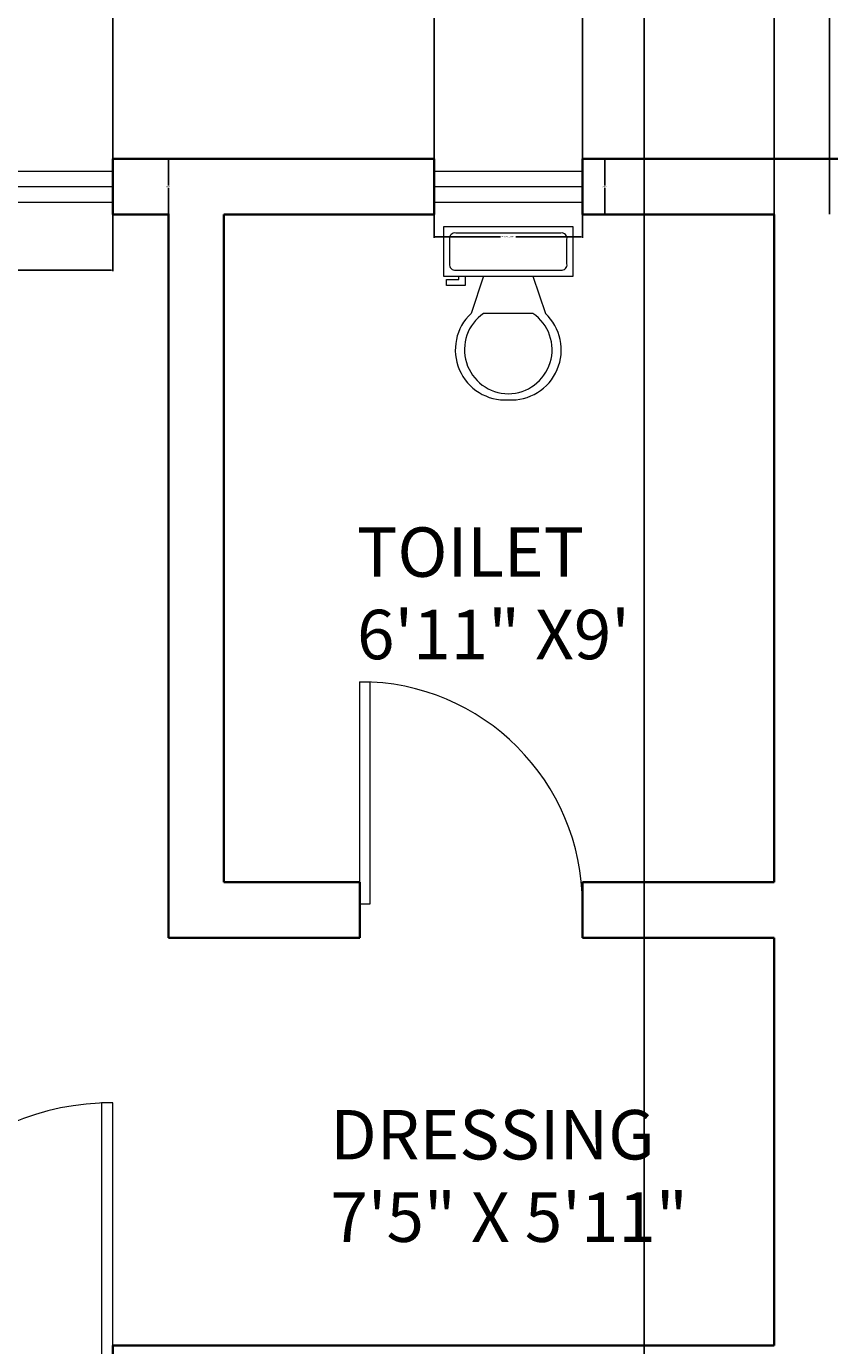
# Model space of a CAD drawing. Units: inches. Extents: x -4843 to -3402, y -164 to 3629.
# Tile 17 of 22: x -4433 to -4303, y 828 to 1042. Entities that reach past the tile are written whole.
import ezdxf

# ---------------------------------------------------------------- set-up
doc = ezdxf.new("R2010")
doc.units = ezdxf.units.IN
for name, color, linetype, lineweight in [('A-ANNO-DIMS', 2, 'Continuous', 18), ('A-AREA-IDEN', 2, 'Continuous', 18), ('doors', 2, 'Continuous', 18), ('toilets', 5, 'Continuous', 18), ('walls', 7, 'Continuous', 35), ('windows', 1, 'Continuous', 18)]:
    doc.layers.add(name, color=color, linetype=linetype, lineweight=lineweight)
doc.styles.get("Standard").update_dxf_attribs({"font": 'arial.ttf'})
doc.dimstyles.get("Standard").update_dxf_attribs({"dimtxt": 0.18, "dimasz": 0.18, "dimexe": 0.18, "dimexo": 0.0625, "dimgap": 0.09, "dimtad": 0, "dimtih": 1, "dimtoh": 1, "dimdec": 4, "dimzin": 0, "dimdsep": 46, "dimtxsty": 'Standard', "dimcen": 0.09, "dimadec": 0, "dimazin": 0, "dimtfac": 1, "dimtdec": 4, "dimtofl": 0, "dimtmove": 0, "dimatfit": 3, "dimfxl": 1, "dimtolj": 1, "dimtzin": 0, "dimarcsym": 0})

# ---------------------------------------------------------------- blocks, each defined once
blk = doc.blocks.new('window')
at = {"layer": 'windows'}
for p, q in [((0, 7), (60, 7)), ((0, 4.5), (60, 4.5)), ((0, 2), (60, 2))]:
    blk.add_line(p, q, dxfattribs=at)
for points in [[(0, 9), (0, 0)], [(60, 0), (60, 9)]]:
    blk.add_lwpolyline(points, dxfattribs=at)
blk = doc.blocks.new('window 2')
at = {"layer": 'windows'}
for p, q in [((0, 8.18), (24, 8.18)), ((0, 5.68), (24, 5.68)), ((0, 3.18), (24, 3.18))]:
    blk.add_line(p, q, dxfattribs=at)
for points in [[(0, 10.18), (0, 1.18)], [(24, 1.18), (24, 10.18)]]:
    blk.add_lwpolyline(points, dxfattribs=at)
blk = doc.blocks.new('*U8')
for p, q in [((0, 0), (0, -6)), ((-40, 0), (-40, -6))]:
    blk.add_line(p, q)
blk.add_lwpolyline([(0, 0), (0, 40), (-1.75, 40), (-1.75, 0)], close=True)
blk.add_arc((0, 0), 40, 90, 180)
blk = doc.blocks.new('*U7')
for p, q in [((0, 0), (0, -6)), ((40, 0), (40, -6))]:
    blk.add_line(p, q)
blk.add_lwpolyline([(0, 0), (0, 40), (1.75, 40), (1.75, 0)], close=True)
blk.add_arc((0, 0), 40, 0, 90)
blk = doc.blocks.new('*U31')
for p, q in [((241.3, -152.4), (241.3, -50.8)), ((-254, -215.9), (-203.2, -215.9)), ((-254, -241.3), (-254, -215.9)), ((-203.2, -215.9), (-203.2, -203.2)), ((-177.8, -203.2), (-177.8, -241.3)), ((-101.6, -203.2), (-152.4, -355.6)), ((101.6, -203.2), (152.4, -355.6)), ((-177.8, -241.3), (-254, -241.3)), ((101.6, -355.6), (-101.6, -355.6))]:
    blk.add_line(p, q)
blk.add_lwpolyline([(266.7, -203.2), (266.7, 0), (-266.7, 0), (-266.7, -203.2)], close=True)
for points in [[(-241.3, -50.8), (-241.3, -152.4)], [(215.9, -25.4), (-215.9, -25.4)], [(-215.9, -177.8), (215.9, -177.8)]]:
    blk.add_lwpolyline(points)
for centre, radius, start, end in [((-219.075, -47.625), 22.45064, 81.8699, 188.1301), ((219.075, -47.625), 22.45064, 351.8699, 98.1301), ((-219.075, -155.575), 22.45064, 171.869898, 278.1301), ((219.075, -155.575), 22.45064, 261.8699, 8.1301), ((-12.12088, -505.93752), 205.61935, 133.01722, 273.38), ((0.94996, -504.77674), 181.02486, 124.50543, 269.7), ((-0.94742, -504.77674), 181.02486, 270.3, 55.4946), ((12.12342, -505.93752), 205.61935, 266.62, 46.9828)]:
    blk.add_arc(centre, radius, start, end)
blk = doc.blocks.new('*D36')
at = {"layer": 'A-ANNO-DIMS', "color": 0, "lineweight": -2, "transparency": 16777216}
for p, q in [((-4478.78, 1011.29), (-4478.78, 1002.17)), ((-4418.78, 1011.29), (-4418.78, 1002.17)), ((-4478.6, 1002.35), (-4450.02, 1002.35)), ((-4418.96, 1002.35), (-4447.55, 1002.35))]:
    blk.add_line(p, q, dxfattribs=at)
at = {"layer": 'A-ANNO-DIMS', "color": 0, "transparency": 16777216}
for points in [[(-4478.6, 1002.38), (-4478.6, 1002.32), (-4478.78, 1002.35)], [(-4418.96, 1002.38), (-4418.96, 1002.32), (-4418.78, 1002.35)]]:
    blk.add_solid(points, dxfattribs=at)
at = {"layer": 'Defpoints', "color": 0, "transparency": 16777216}
for p in [(-4478.78, 1011.35), (-4418.78, 1011.35), (-4418.78, 1002.35)]:
    blk.add_point(p, dxfattribs=at)
at = {"layer": 'A-ANNO-DIMS', "color": 0, "transparency": 16777216, "insert": (-4448.78, 1002.35), "char_height": 0.18, "attachment_point": 5}
blk.add_mtext('\\A1;WINDOW A 60 TYP.', dxfattribs=at)
blk = doc.blocks.new('*D37')
at = {"layer": 'A-ANNO-DIMS', "color": 0, "lineweight": -2, "transparency": 16777216}
for p, q in [((-4418.72, 1020.35), (-4409.6, 1020.35)), ((-4409.78, 1020.17), (-4409.78, 1016.04)), ((-4409.78, 1011.53), (-4409.78, 1015.67)), ((-4418.72, 1011.35), (-4409.6, 1011.35))]:
    blk.add_line(p, q, dxfattribs=at)
at = {"layer": 'A-ANNO-DIMS', "color": 0, "transparency": 16777216}
for points in [[(-4409.81, 1020.17), (-4409.75, 1020.17), (-4409.78, 1020.35)], [(-4409.81, 1011.53), (-4409.75, 1011.53), (-4409.78, 1011.35)]]:
    blk.add_solid(points, dxfattribs=at)
at = {"layer": 'Defpoints', "color": 0, "transparency": 16777216}
for p in [(-4418.78, 1020.35), (-4409.78, 1020.35), (-4418.78, 1011.35)]:
    blk.add_point(p, dxfattribs=at)
at = {"layer": 'A-ANNO-DIMS', "color": 0, "transparency": 16777216, "insert": (-4409.78, 1015.85), "char_height": 0.18, "attachment_point": 5}
blk.add_mtext('\\A1;9 TYP.', dxfattribs=at)
blk = doc.blocks.new('*D40')
at = {"layer": 'A-ANNO-DIMS', "color": 0, "lineweight": -2, "transparency": 16777216}
for p, q in [((-4366.78, 1011.29), (-4366.78, 1007.57)), ((-4342.78, 1011.29), (-4342.78, 1007.57)), ((-4366.6, 1007.75), (-4356.03, 1007.75)), ((-4342.96, 1007.75), (-4353.54, 1007.75))]:
    blk.add_line(p, q, dxfattribs=at)
at = {"layer": 'A-ANNO-DIMS', "color": 0, "transparency": 16777216}
for points in [[(-4366.6, 1007.78), (-4366.6, 1007.72), (-4366.78, 1007.75)], [(-4342.96, 1007.78), (-4342.96, 1007.72), (-4342.78, 1007.75)]]:
    blk.add_solid(points, dxfattribs=at)
at = {"layer": 'Defpoints', "color": 0, "transparency": 16777216}
for p in [(-4366.78, 1011.35), (-4342.78, 1011.35), (-4342.78, 1007.75)]:
    blk.add_point(p, dxfattribs=at)
at = {"layer": 'A-ANNO-DIMS', "color": 0, "transparency": 16777216, "insert": (-4354.78, 1007.75), "char_height": 0.18, "attachment_point": 5}
blk.add_mtext('\\A1;WINDOW C 24 TYP.', dxfattribs=at)
blk = doc.blocks.new('*D41')
at = {"layer": 'A-ANNO-DIMS', "color": 0, "lineweight": -2, "transparency": 16777216}
for p, q in [((-4342.72, 1020.35), (-4339, 1020.35)), ((-4339.18, 1020.17), (-4339.18, 1016.04)), ((-4339.18, 1011.53), (-4339.18, 1015.67)), ((-4342.72, 1011.35), (-4339, 1011.35))]:
    blk.add_line(p, q, dxfattribs=at)
at = {"layer": 'A-ANNO-DIMS', "color": 0, "transparency": 16777216}
for points in [[(-4339.21, 1020.17), (-4339.15, 1020.17), (-4339.18, 1020.35)], [(-4339.21, 1011.53), (-4339.15, 1011.53), (-4339.18, 1011.35)]]:
    blk.add_solid(points, dxfattribs=at)
at = {"layer": 'Defpoints', "color": 0, "transparency": 16777216}
for p in [(-4342.78, 1020.35), (-4339.18, 1020.35), (-4342.78, 1011.35)]:
    blk.add_point(p, dxfattribs=at)
at = {"layer": 'A-ANNO-DIMS', "color": 0, "transparency": 16777216, "insert": (-4339.18, 1015.85), "char_height": 0.18, "attachment_point": 5}
blk.add_mtext('\\A1;9 TYP.', dxfattribs=at)
blk = doc.blocks.new('*D70')
at = {"layer": 'A-ANNO-DIMS', "color": 0, "lineweight": -2, "transparency": 16777216}
for p, q in [((-4418.78, 1020.42), (-4418.78, 1392.95)), ((-4418.6, 1392.77), (-4393, 1392.77)), ((-4366.96, 1392.77), (-4392.56, 1392.77)), ((-4366.78, 1020.42), (-4366.78, 1392.95))]:
    blk.add_line(p, q, dxfattribs=at)
at = {"layer": 'A-ANNO-DIMS', "color": 0, "transparency": 16777216}
for points in [[(-4418.6, 1392.8), (-4418.6, 1392.74), (-4418.78, 1392.77)], [(-4366.96, 1392.8), (-4366.96, 1392.74), (-4366.78, 1392.77)]]:
    blk.add_solid(points, dxfattribs=at)
at = {"layer": 'Defpoints', "color": 0, "transparency": 16777216}
for p in [(-4366.78, 1392.77), (-4418.78, 1020.35), (-4366.78, 1020.35)]:
    blk.add_point(p, dxfattribs=at)
at = {"layer": 'A-ANNO-DIMS', "color": 0, "transparency": 16777216, "insert": (-4392.78, 1392.77), "char_height": 0.18, "attachment_point": 5}
blk.add_mtext('\\A1;52', dxfattribs=at)
blk = doc.blocks.new('*D71')
at = {"layer": 'A-ANNO-DIMS', "color": 0, "lineweight": -2, "transparency": 16777216}
for p, q in [((-4342.78, 1020.42), (-4342.78, 1392.95)), ((-4342.6, 1392.77), (-4327.48, 1392.77)), ((-4311.96, 1392.77), (-4327.08, 1392.77)), ((-4311.78, 1011.42), (-4311.78, 1392.95))]:
    blk.add_line(p, q, dxfattribs=at)
at = {"layer": 'A-ANNO-DIMS', "color": 0, "transparency": 16777216}
for points in [[(-4342.6, 1392.8), (-4342.6, 1392.74), (-4342.78, 1392.77)], [(-4311.96, 1392.8), (-4311.96, 1392.74), (-4311.78, 1392.77)]]:
    blk.add_solid(points, dxfattribs=at)
at = {"layer": 'Defpoints', "color": 0, "transparency": 16777216}
for p in [(-4311.78, 1392.77), (-4342.78, 1020.35), (-4311.78, 1011.35)]:
    blk.add_point(p, dxfattribs=at)
at = {"layer": 'A-ANNO-DIMS', "color": 0, "transparency": 16777216, "insert": (-4327.28, 1392.77), "char_height": 0.18, "attachment_point": 5}
blk.add_mtext('\\A1;31', dxfattribs=at)
blk = doc.blocks.new('*D72')
at = {"layer": 'A-ANNO-DIMS', "color": 0, "lineweight": -2, "transparency": 16777216}
for p, q in [((-4302.78, 1011.42), (-4302.78, 1392.95)), ((-4302.6, 1392.77), (-4285, 1392.77)), ((-4266.96, 1392.77), (-4284.56, 1392.77)), ((-4266.78, 1020.42), (-4266.78, 1392.95))]:
    blk.add_line(p, q, dxfattribs=at)
at = {"layer": 'A-ANNO-DIMS', "color": 0, "transparency": 16777216}
for points in [[(-4302.6, 1392.8), (-4302.6, 1392.74), (-4302.78, 1392.77)], [(-4266.96, 1392.8), (-4266.96, 1392.74), (-4266.78, 1392.77)]]:
    blk.add_solid(points, dxfattribs=at)
at = {"layer": 'Defpoints', "color": 0, "transparency": 16777216}
for p in [(-4266.78, 1392.77), (-4266.78, 1020.35), (-4302.78, 1011.35)]:
    blk.add_point(p, dxfattribs=at)
at = {"layer": 'A-ANNO-DIMS', "color": 0, "transparency": 16777216, "insert": (-4284.78, 1392.77), "char_height": 0.18, "attachment_point": 5}
blk.add_mtext('\\A1;36', dxfattribs=at)
blk = doc.blocks.new('*D81')
at = {"layer": 'A-ANNO-DIMS', "color": 0, "lineweight": -2, "transparency": 16777216}
for p, q in [((-4332.78, 86.42), (-4332.78, 1392.95)), ((-4332.6, 1392.77), (-4168.61, 1392.77)), ((-4003.86, 1392.77), (-4167.86, 1392.77)), ((-4003.68, 86.42), (-4003.68, 1392.95))]:
    blk.add_line(p, q, dxfattribs=at)
at = {"layer": 'A-ANNO-DIMS', "color": 0, "transparency": 16777216}
for points in [[(-4332.6, 1392.8), (-4332.6, 1392.74), (-4332.78, 1392.77)], [(-4003.86, 1392.8), (-4003.86, 1392.74), (-4003.68, 1392.77)]]:
    blk.add_solid(points, dxfattribs=at)
at = {"layer": 'Defpoints', "color": 0, "transparency": 16777216}
for p in [(-4003.68, 1392.77), (-4332.78, 86.35), (-4003.68, 86.35)]:
    blk.add_point(p, dxfattribs=at)
at = {"layer": 'A-ANNO-DIMS', "color": 0, "transparency": 16777216, "insert": (-4168.23, 1392.77), "char_height": 0.18, "attachment_point": 5}
blk.add_mtext('\\A1;329.1', dxfattribs=at)

msp = doc.modelspace()

# ---------------------------------------------------------------- linework, layer by layer
at = {"layer": 'walls'}
for p, q in [((-4418.78, 1020.35), (-4366.78, 1020.35)), ((-4342.78, 1020.35), (-4266.78, 1020.35)), ((-4418.78, 1011.35), (-4409.78, 1011.35)), ((-4409.78, 1011.35), (-4409.78, 894.35)), ((-4400.78, 1011.35), (-4400.78, 903.35)), ((-4400.78, 1011.35), (-4366.78, 1011.35)), ((-4342.78, 1011.35), (-4311.78, 1011.35)), ((-4311.78, 1011.35), (-4311.78, 903.35)), ((-4400.78, 903.35), (-4378.78, 903.35)), ((-4342.78, 903.35), (-4311.78, 903.35)), ((-4409.78, 894.35), (-4378.78, 894.35)), ((-4342.78, 894.35), (-4311.78, 894.35)), ((-4311.78, 894.35), (-4311.78, 828.35)), ((-4418.78, 828.35), (-4311.78, 828.35))]:
    msp.add_line(p, q, dxfattribs=at)
for points in [[(-4418.78, 1011.35), (-4418.78, 1020.35)], [(-4366.78, 1020.35), (-4366.78, 1011.35)], [(-4342.78, 1011.35), (-4342.78, 1020.35)], [(-4378.78, 894.35), (-4378.78, 903.35)], [(-4342.78, 903.35), (-4342.78, 894.35)], [(-4418.78, 819.35), (-4418.78, 828.35)]]:
    msp.add_lwpolyline(points, dxfattribs=at)

# ---------------------------------------------------------------- block references
at = {"layer": 'doors'}
for name, p, xscale, yscale, zscale in [('*U7', (-4378.78, 899.75), 0.9, 0.9, 0.9), ('*U8', (-4418.78, 825.65), 1.05, 1.05, 1.05)]:
    msp.add_blockref(name, p, dxfattribs=dict(at, xscale=xscale, yscale=yscale, zscale=zscale))
at = {"layer": 'toilets', "xscale": 0.0393700787401575, "yscale": 0.0393700787401575, "zscale": 0.0393700787401575}
msp.add_blockref('*U31', (-4354.78, 1009.35), dxfattribs=at)
at = {"layer": 'windows'}
for name, p in [('window', (-4478.78, 1011.35)), ('window 2', (-4366.78, 1010.17))]:
    msp.add_blockref(name, p, dxfattribs=at)

# ---------------------------------------------------------------- texts
at = {"layer": 'A-AREA-IDEN', "char_height": 8, "attachment_point": 1}
for s, insert in [('TOILET\\P6\'11" X9\'', (-4379.25, 960.73)), ('DRESSING\\P7\'5" X 5\'11"', (-4383.57, 866.47))]:
    msp.add_mtext_dynamic_manual_height_columns(s, width=66.873, gutter_width=60, heights=[0], dxfattribs=dict(at, insert=insert))

# ---------------------------------------------------------------- dimensions: what is measured, and where the dimension line sits
at = {"layer": 'A-ANNO-DIMS'}
for base, p1, p2, override, picture, middle in [((-4366.78, 1392.77), (-4418.78, 1020.35), (-4366.78, 1020.35), {"dimdec": 0, "dimlfac": 1, "dimrnd": 0, "dimzin": 0, "dimdsep": 46, "dimlunit": 2}, '*D70', (-4392.78, 1392.77)), ((-4311.78, 1392.77), (-4342.78, 1020.35), (-4311.78, 1011.35), {"dimdec": 0, "dimlfac": 1, "dimrnd": 0, "dimzin": 0, "dimdsep": 46, "dimlunit": 2}, '*D71', (-4327.28, 1392.77)), ((-4003.68, 1392.77), (-4332.78, 86.35), (-4003.68, 86.35), {"dimdec": 1, "dimlfac": 1, "dimrnd": 0, "dimzin": 0, "dimdsep": 46, "dimlunit": 2}, '*D81', (-4168.23, 1392.77)), ((-4266.78, 1392.77), (-4302.78, 1011.35), (-4266.78, 1020.35), {"dimdec": 0, "dimlfac": 1, "dimrnd": 0, "dimzin": 0, "dimdsep": 46, "dimlunit": 2}, '*D72', (-4284.78, 1392.77))]:
    dim = msp.add_linear_dim(base=base, p1=p1, p2=p2, dimstyle='Standard', override=override, dxfattribs=at)
    dim.commit()
    dim.dimension.update_dxf_attribs({"geometry": picture, "text_midpoint": middle})
for base, p1, p2, picture, middle in [((-4409.78, 1020.35), (-4418.78, 1011.35), (-4418.78, 1020.35), '*D37', (-4409.78, 1015.85)), ((-4339.18, 1020.35), (-4342.78, 1011.35), (-4342.78, 1020.35), '*D41', (-4339.18, 1015.85))]:
    dim = msp.add_linear_dim(base=base, p1=p1, p2=p2, angle=90, text='<> TYP.', dimstyle='Standard', override={"dimdec": 0, "dimlfac": 1, "dimrnd": 0, "dimzin": 0, "dimdsep": 46, "dimlunit": 2}, dxfattribs=at)
    dim.commit()
    dim.dimension.update_dxf_attribs({"geometry": picture, "text_midpoint": middle})
for base, p1, p2, text, picture, middle in [((-4418.78, 1002.35), (-4478.78, 1011.35), (-4418.78, 1011.35), 'WINDOW A <> TYP.', '*D36', (-4448.78, 1002.35)), ((-4342.78, 1007.75), (-4366.78, 1011.35), (-4342.78, 1011.35), 'WINDOW C <> TYP.', '*D40', (-4354.78, 1007.75))]:
    dim = msp.add_linear_dim(base=base, p1=p1, p2=p2, text=text, dimstyle='Standard', override={"dimdec": 0, "dimlfac": 1, "dimrnd": 0, "dimzin": 0, "dimdsep": 46, "dimlunit": 2}, dxfattribs=at)
    dim.commit()
    dim.dimension.update_dxf_attribs({"geometry": picture, "text_midpoint": middle})

doc.saveas('drawing.dxf')
